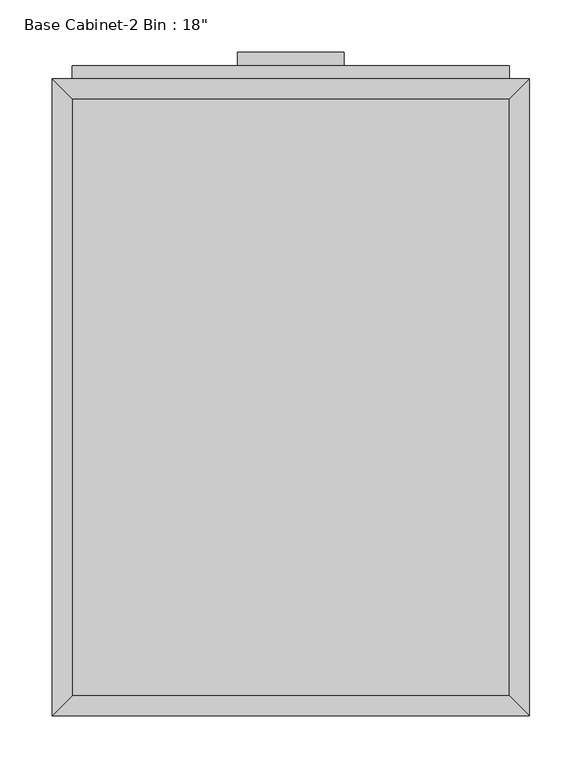
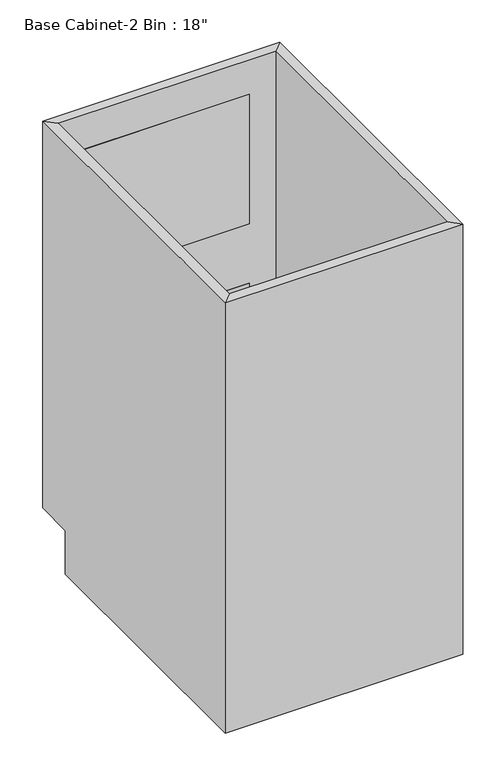
"""IFC4 building model written with IfcOpenShell, lengths in millimetres: furniture geometry."""

from ifc_helpers import new_model, si_unit, frame, origin, place, context, project, spatial, polyline, outline, extrude, faceted_brep, source, transform, mapped, element, save


def furniture_3a47f844(model_context):
    return source(origin(), model_context, "Body", "SolidModel", [
        extrude(outline(polyline([(69.5377049, 635.0), (69.5377049, 622.3), (-32.0622951, 622.3), (-32.0622951, 635.0), (69.5377049, 635.0)])), frame((0.0, 0.0, 819.15), z_axis=(0.0, 0.0, 1.0), x_axis=(1.0, 0.0, 0.0)), (0.0, 0.0, 1.0), 12.7),
        extrude(outline(polyline([(69.5377049, 635.0), (69.5377049, 622.3), (-32.0622951, 622.3), (-32.0622951, 635.0), (69.5377049, 635.0)])), frame((0.0, 0.0, 434.975), z_axis=(0.0, 0.0, 1.0), x_axis=(1.0, 0.0, 0.0)), (0.0, 0.0, 1.0), 12.7),
        extrude(outline(polyline([(857.25, 228.2877049), (857.25, -190.8122951), (492.125, -190.8122951), (492.125, 228.2877049), (857.25, 228.2877049)]), holes=[polyline([(806.45, 177.4877049), (542.925, 177.4877049), (542.925, -140.0122951), (806.45, -140.0122951), (806.45, 177.4877049)])]), frame((0.0, 609.6, 0.0), z_axis=(0.0, 1.0, 0.0), x_axis=(0.0, 0.0, 1.0)), (0.0, 0.0, 1.0), 12.7),
        extrude(outline(polyline([(473.075, 228.2877049), (473.075, -190.8122951), (107.95, -190.8122951), (107.95, 228.2877049), (473.075, 228.2877049)]), holes=[polyline([(422.275, 177.4877049), (158.75, 177.4877049), (158.75, -140.0122951), (422.275, -140.0122951), (422.275, 177.4877049)])]), frame((0.0, 609.6, 0.0), z_axis=(0.0, 1.0, 0.0), x_axis=(0.0, 0.0, 1.0)), (0.0, 0.0, 1.0), 12.7),
        extrude(outline(polyline([(177.4877049, 609.6), (177.4877049, 590.55), (-140.0122951, 590.55), (-140.0122951, 609.6), (177.4877049, 609.6)])), frame((0.0, 0.0, 542.925), z_axis=(0.0, 0.0, 1.0), x_axis=(1.0, 0.0, 0.0)), (0.0, 0.0, 1.0), 263.525),
        extrude(outline(polyline([(177.4877049, 609.6), (177.4877049, 590.55), (-140.0122951, 590.55), (-140.0122951, 609.6), (177.4877049, 609.6)])), frame((0.0, 0.0, 158.75), z_axis=(0.0, 0.0, 1.0), x_axis=(1.0, 0.0, 0.0)), (0.0, 0.0, 1.0), 263.525),
        extrude(outline(polyline([(228.2877049, 19.05), (-190.8122951, 19.05), (-190.8122951, 590.55), (228.2877049, 590.55), (228.2877049, 19.05)])), frame((0.0, 0.0, 88.9), z_axis=(0.0, 0.0, 1.0), x_axis=(1.0, 0.0, 0.0)), (0.0, 0.0, 1.0), 19.05),
        faceted_brep([(228.2877049, 590.55, 876.3), (-190.8122951, 590.55, 876.3), (-190.8122951, 590.55, 88.9), (228.2877049, 590.55, 88.9), (177.4877049, 590.55, 542.925), (-140.0122951, 590.55, 542.925), (-140.0122951, 590.55, 806.45), (177.4877049, 590.55, 806.45), (177.4877049, 590.55, 158.75), (-140.0122951, 590.55, 158.75), (-140.0122951, 590.55, 422.275), (177.4877049, 590.55, 422.275), (247.3377049, 609.6, 876.3), (-209.8622951, 609.6, 876.3), (247.3377049, 609.6, 88.9), (-209.8622951, 609.6, 88.9), (177.4877049, 609.6, 806.45), (-140.0122951, 609.6, 806.45), (-140.0122951, 609.6, 542.925), (177.4877049, 609.6, 542.925), (177.4877049, 609.6, 422.275), (-140.0122951, 609.6, 422.275), (-140.0122951, 609.6, 158.75), (177.4877049, 609.6, 158.75), (-190.8122951, 19.05, 876.3), (-190.8122951, 19.05, 88.9), (-190.8122951, 533.4, 88.9), (-209.8622951, 0.0, 876.3), (-209.8622951, 533.4, 88.9), (-209.8622951, 533.4, 0.0), (-209.8622951, 0.0, 0.0), (228.2877049, 19.05, 876.3), (228.2877049, 19.05, 88.9), (247.3377049, 0.0, 876.3), (247.3377049, 0.0, 0.0), (228.2877049, 533.4, 88.9), (247.3377049, 533.4, 0.0), (247.3377049, 533.4, 88.9)], [[[0, 1, 2, 3], [4, 5, 6, 7], [8, 9, 10, 11]], [[0, 12, 13, 1]], [[12, 14, 15, 13], [16, 17, 18, 19], [20, 21, 22, 23]], [[2, 15, 14, 3]], [[1, 24, 25, 26, 2]], [[13, 27, 24, 1]], [[15, 28, 29, 30, 27, 13]], [[2, 26, 28, 15]], [[24, 31, 32, 25]], [[27, 33, 31, 24]], [[27, 30, 34, 33]], [[3, 35, 32, 31, 0]], [[0, 31, 33, 12]], [[12, 33, 34, 36, 37, 14]], [[14, 37, 35, 3]], [[26, 25, 32, 35]], [[34, 30, 29, 36]], [[29, 28, 26, 35, 37, 36]], [[4, 7, 16, 19]], [[19, 18, 5, 4]], [[18, 17, 6, 5]], [[7, 6, 17, 16]], [[8, 11, 20, 23]], [[23, 22, 9, 8]], [[22, 21, 10, 9]], [[11, 10, 21, 20]]]),
    ])


if __name__ == "__main__":
    model = new_model("IFC4")
    model_context = context("Model", 3, world=origin())
    ifc_project = project(units=[si_unit("LENGTHUNIT", "METRE", prefix="MILLI")], contexts=[model_context])
    site = spatial("IfcSite", under=ifc_project)
    building = spatial("IfcBuilding", under=site)
    placement = place(None, origin())
    furniture_shape = furniture_3a47f844(model_context)
    element("IfcFurniture", 1, ObjectType="Base Cabinet-2 Bin : 18\"", at=placement, inside=building, context=model_context, shape_type="MappedRepresentation", body=[
        mapped(furniture_shape, transform((0.0, 0.0, 0.0), x_axis=(1.0, 0.0, 0.0), y_axis=(0.0, 1.0, 0.0), z_axis=(0.0, 0.0, 1.0))),
    ])
    save(model, "model.ifc")

# Revit data of these elements
# Type "Base Cabinet-2 Bin : 18\""
#   Assembly Code = "C1030410"
#   Depth = 2' - 0"
#   Height = 2' - 10 1/2"
#   Toe Depth = 0' - 3"
#   Toe Height = 0' - 3 1/2"
#   Width = 1' - 6"
#   Cabinet Material = none
#   Door/Drawer Material = none
#   Handle Material = Cabinets - Handles
#   Panels = none
#   Default Elevation = 0
# Element 1 (IfcFurniture, "Base Cabinet-2 Bin : 18\"")
#   Materials on its faces: "Cabinets", "Cabinets - Handles", "Cabinets - Panel/Glass"
# Materials
#   "Cabinets - Handles": class "Metal", colour RGB 57 57 57, transparency 0
#   "Cabinets": colour RGB 249 249 249, transparency 0
#   "Cabinets - Panel/Glass": colour RGB 252 255 255, transparency 0.72
